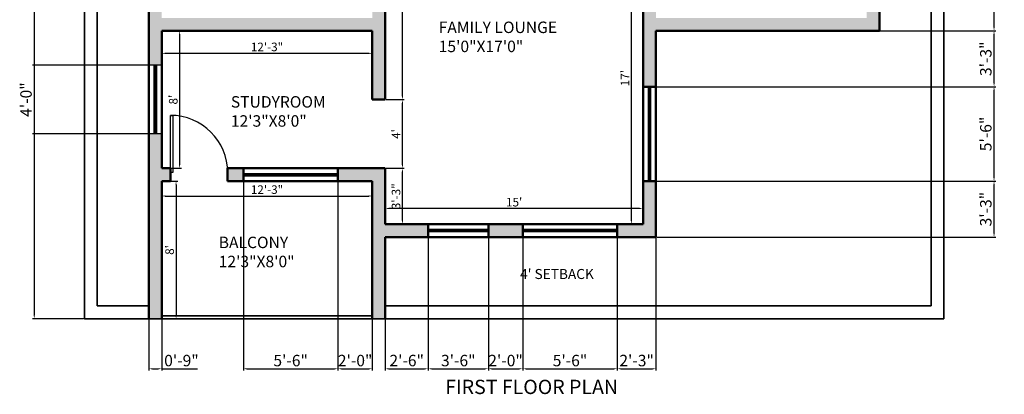
# Model space of a CAD drawing. Units: inches. Extents: x 2442 to 3851, y 589 to 2836.
# Tile 18 of 22: x 3164 to 3851, y 2138 to 2400. Entities that reach past the tile are written whole.
import ezdxf

# ---------------------------------------------------------------- set-up
doc = ezdxf.new("R2010")
doc.units = ezdxf.units.IN
for name, color, linetype, lineweight in [('A-ANNO-DIMS', 2, 'Continuous', 18), ('A-ANNO-TEXT', 7, 'Continuous', 18), ('A-AREA-IDEN', 7, 'Continuous', 18), ('A-DOOR', 4, 'Continuous', 25), ('A-GLAZ', 1, 'Continuous', 25), ('A-WALL', 7, 'Continuous', 50), ('A-WALL-PATT', 8, 'Continuous', 13), ('C-PROP', 7, 'Continuous', 35)]:
    doc.layers.add(name, color=color, linetype=linetype, lineweight=lineweight)
doc.styles.get("Standard").update_dxf_attribs({"font": 'arial.ttf'})
doc.dimstyles.new('ISO-25', dxfattribs={"dimtxt": 8, "dimasz": 2.5, "dimexe": 1.25, "dimexo": 0.625, "dimtad": 1, "dimlunit": 3, "dimtxsty": 'Standard', "dimcen": 2.5, "dimadec": 0, "dimazin": 0, "dimtfac": 1, "dimtmove": 0, "dimatfit": 3, "dimfxl": 1, "dimarcsym": 0})

# ---------------------------------------------------------------- blocks, each defined once
blk = doc.blocks.new('*U22')
for p, q in [((0, 0), (0, -6)), ((40, 0), (40, -6))]:
    blk.add_line(p, q)
blk.add_lwpolyline([(0, 0), (0, 40), (1.75, 40), (1.75, 0)], close=True)
blk.add_arc((0, 0), 40, 0, 90)
blk = doc.blocks.new('*D93')
at = {"layer": 'A-ANNO-DIMS', "color": 0, "lineweight": -2, "transparency": 16777216}
for p, q in [((3263.65, 2287.21), (3274.25, 2287.21)), ((3273, 2284.71), (3273, 2193.71)), ((3263.65, 2191.21), (3274.25, 2191.21))]:
    blk.add_line(p, q, dxfattribs=at)
at = {"layer": 'A-ANNO-DIMS', "color": 0, "transparency": 16777216}
for points in [[(3272.58, 2284.71), (3273.42, 2284.71), (3273, 2287.21)], [(3272.58, 2193.71), (3273.42, 2193.71), (3273, 2191.21)]]:
    blk.add_solid(points, dxfattribs=at)
at = {"layer": 'Defpoints', "color": 0, "transparency": 16777216}
for p in [(3263.02, 2287.21), (3263.02, 2191.21), (3273, 2191.21)]:
    blk.add_point(p, dxfattribs=at)
at = {"layer": 'A-ANNO-DIMS', "color": 0, "transparency": 16777216, "insert": (3269.31, 2239.21), "char_height": 6, "attachment_point": 5, "rotation": 90}
blk.add_mtext("8'", dxfattribs=at)
blk = doc.blocks.new('*D94')
at = {"layer": 'A-ANNO-DIMS', "color": 0, "lineweight": -2, "transparency": 16777216}
for p, q in [((3263.02, 2286.58), (3263.02, 2275.62)), ((3410.02, 2286.58), (3410.02, 2275.62)), ((3265.52, 2276.87), (3407.52, 2276.87))]:
    blk.add_line(p, q, dxfattribs=at)
at = {"layer": 'A-ANNO-DIMS', "color": 0, "transparency": 16777216}
for points in [[(3265.52, 2277.29), (3265.52, 2276.45), (3263.02, 2276.87)], [(3407.52, 2277.29), (3407.52, 2276.45), (3410.02, 2276.87)]]:
    blk.add_solid(points, dxfattribs=at)
at = {"layer": 'Defpoints', "color": 0, "transparency": 16777216}
for p in [(3263.02, 2287.21), (3410.02, 2287.21), (3410.02, 2276.87)]:
    blk.add_point(p, dxfattribs=at)
at = {"layer": 'A-ANNO-DIMS', "color": 0, "transparency": 16777216, "insert": (3336.52, 2280.56), "char_height": 6, "attachment_point": 5}
blk.add_mtext('12\'-3"', dxfattribs=at)
blk = doc.blocks.new('*D95')
at = {"layer": 'A-ANNO-DIMS', "color": 0, "lineweight": -2, "transparency": 16777216}
for p, q in [((3419.65, 2296.21), (3432.29, 2296.21)), ((3431.04, 2259.71), (3431.04, 2293.71)), ((3419.65, 2257.21), (3432.29, 2257.21))]:
    blk.add_line(p, q, dxfattribs=at)
at = {"layer": 'A-ANNO-DIMS', "color": 0, "transparency": 16777216}
for points in [[(3430.63, 2293.71), (3431.46, 2293.71), (3431.04, 2296.21)], [(3430.63, 2259.71), (3431.46, 2259.71), (3431.04, 2257.21)]]:
    blk.add_solid(points, dxfattribs=at)
at = {"layer": 'Defpoints', "color": 0, "transparency": 16777216}
for p in [(3419.02, 2296.21), (3431.04, 2296.21), (3419.02, 2257.21)]:
    blk.add_point(p, dxfattribs=at)
at = {"layer": 'A-ANNO-DIMS', "color": 0, "transparency": 16777216, "insert": (3427.35, 2276.71), "char_height": 6, "attachment_point": 5, "rotation": 90}
blk.add_mtext('3\'-3"', dxfattribs=at)
blk = doc.blocks.new('*D96')
at = {"layer": 'A-ANNO-DIMS', "color": 0, "lineweight": -2, "transparency": 16777216}
for p, q in [((3419.65, 2344.21), (3432.29, 2344.21)), ((3431.04, 2298.71), (3431.04, 2341.71)), ((3419.65, 2296.21), (3432.29, 2296.21))]:
    blk.add_line(p, q, dxfattribs=at)
at = {"layer": 'A-ANNO-DIMS', "color": 0, "transparency": 16777216}
for points in [[(3430.63, 2341.71), (3431.46, 2341.71), (3431.04, 2344.21)], [(3430.63, 2298.71), (3431.46, 2298.71), (3431.04, 2296.21)]]:
    blk.add_solid(points, dxfattribs=at)
at = {"layer": 'Defpoints', "color": 0, "transparency": 16777216}
for p in [(3419.02, 2344.21), (3431.04, 2344.21), (3419.02, 2296.21)]:
    blk.add_point(p, dxfattribs=at)
at = {"layer": 'A-ANNO-DIMS', "color": 0, "transparency": 16777216, "insert": (3427.42, 2320.21), "char_height": 6, "attachment_point": 5, "rotation": 90}
blk.add_mtext("4'", dxfattribs=at)
blk = doc.blocks.new('*D97')
at = {"layer": 'A-ANNO-DIMS', "color": 0, "lineweight": -2, "transparency": 16777216}
for p, q in [((3419.65, 2506.21), (3432.29, 2506.21)), ((3431.04, 2346.71), (3431.04, 2503.71)), ((3419.65, 2344.21), (3432.29, 2344.21))]:
    blk.add_line(p, q, dxfattribs=at)
at = {"layer": 'A-ANNO-DIMS', "color": 0, "transparency": 16777216}
for points in [[(3430.63, 2503.71), (3431.46, 2503.71), (3431.04, 2506.21)], [(3430.63, 2346.71), (3431.46, 2346.71), (3431.04, 2344.21)]]:
    blk.add_solid(points, dxfattribs=at)
at = {"layer": 'Defpoints', "color": 0, "transparency": 16777216}
for p in [(3419.02, 2506.21), (3431.04, 2506.21), (3419.02, 2344.21)]:
    blk.add_point(p, dxfattribs=at)
at = {"layer": 'A-ANNO-DIMS', "color": 0, "transparency": 16777216, "insert": (3427.35, 2425.21), "char_height": 6, "attachment_point": 5, "rotation": 90}
blk.add_mtext('13\'-6"', dxfattribs=at)
blk = doc.blocks.new('*D130')
at = {"layer": 'A-ANNO-DIMS', "color": 0, "lineweight": -2, "transparency": 16777216}
for p, q in [((3263.02, 2391.58), (3263.02, 2375.27)), ((3410.02, 2391.58), (3410.02, 2375.27)), ((3265.52, 2376.52), (3407.52, 2376.52))]:
    blk.add_line(p, q, dxfattribs=at)
at = {"layer": 'A-ANNO-DIMS', "color": 0, "transparency": 16777216}
for points in [[(3265.52, 2376.94), (3265.52, 2376.11), (3263.02, 2376.52)], [(3407.52, 2376.94), (3407.52, 2376.11), (3410.02, 2376.52)]]:
    blk.add_solid(points, dxfattribs=at)
at = {"layer": 'Defpoints', "color": 0, "transparency": 16777216}
for p in [(3263.02, 2392.21), (3410.02, 2392.21), (3410.02, 2376.52)]:
    blk.add_point(p, dxfattribs=at)
at = {"layer": 'A-ANNO-DIMS', "color": 0, "transparency": 16777216, "insert": (3336.52, 2380.21), "char_height": 6, "attachment_point": 5}
blk.add_mtext('12\'-3"', dxfattribs=at)
blk = doc.blocks.new('*D131')
at = {"layer": 'A-ANNO-DIMS', "color": 0, "lineweight": -2, "transparency": 16777216}
for p, q in [((3263.65, 2392.21), (3276.76, 2392.21)), ((3275.51, 2389.71), (3275.51, 2298.71)), ((3263.65, 2296.21), (3276.76, 2296.21))]:
    blk.add_line(p, q, dxfattribs=at)
at = {"layer": 'A-ANNO-DIMS', "color": 0, "transparency": 16777216}
for points in [[(3275.1, 2389.71), (3275.93, 2389.71), (3275.51, 2392.21)], [(3275.1, 2298.71), (3275.93, 2298.71), (3275.51, 2296.21)]]:
    blk.add_solid(points, dxfattribs=at)
at = {"layer": 'Defpoints', "color": 0, "transparency": 16777216}
for p in [(3263.02, 2392.21), (3263.02, 2296.21), (3275.51, 2296.21)]:
    blk.add_point(p, dxfattribs=at)
at = {"layer": 'A-ANNO-DIMS', "color": 0, "transparency": 16777216, "insert": (3271.82, 2344.21), "char_height": 6, "attachment_point": 5, "rotation": 90}
blk.add_mtext("8'", dxfattribs=at)
blk = doc.blocks.new('*D132')
at = {"layer": 'A-ANNO-DIMS', "color": 0, "lineweight": -2, "transparency": 16777216}
for p, q in [((3419.02, 2257.83), (3419.02, 2269.37)), ((3599.02, 2257.83), (3599.02, 2269.37)), ((3596.52, 2268.12), (3421.52, 2268.12))]:
    blk.add_line(p, q, dxfattribs=at)
at = {"layer": 'A-ANNO-DIMS', "color": 0, "transparency": 16777216}
for points in [[(3421.52, 2268.54), (3421.52, 2267.7), (3419.02, 2268.12)], [(3596.52, 2268.54), (3596.52, 2267.7), (3599.02, 2268.12)]]:
    blk.add_solid(points, dxfattribs=at)
at = {"layer": 'Defpoints', "color": 0, "transparency": 16777216}
for p in [(3419.02, 2268.12), (3419.02, 2257.21), (3599.02, 2257.21)]:
    blk.add_point(p, dxfattribs=at)
at = {"layer": 'A-ANNO-DIMS', "color": 0, "transparency": 16777216, "insert": (3509.02, 2271.81), "char_height": 6, "attachment_point": 5}
blk.add_mtext("15'", dxfattribs=at)
blk = doc.blocks.new('*D133')
at = {"layer": 'A-ANNO-DIMS', "color": 0, "lineweight": -2, "transparency": 16777216}
for p, q in [((3598.4, 2461.21), (3589.59, 2461.21)), ((3590.84, 2259.71), (3590.84, 2458.71)), ((3598.4, 2257.21), (3589.59, 2257.21))]:
    blk.add_line(p, q, dxfattribs=at)
at = {"layer": 'A-ANNO-DIMS', "color": 0, "transparency": 16777216}
for points in [[(3590.43, 2458.71), (3591.26, 2458.71), (3590.84, 2461.21)], [(3590.43, 2259.71), (3591.26, 2259.71), (3590.84, 2257.21)]]:
    blk.add_solid(points, dxfattribs=at)
at = {"layer": 'Defpoints', "color": 0, "transparency": 16777216}
for p in [(3590.84, 2461.21), (3599.02, 2461.21), (3599.02, 2257.21)]:
    blk.add_point(p, dxfattribs=at)
at = {"layer": 'A-ANNO-DIMS', "color": 0, "transparency": 16777216, "insert": (3587.21, 2359.21), "char_height": 6, "attachment_point": 5, "rotation": 90}
blk.add_mtext("17'", dxfattribs=at)
blk = doc.blocks.new('*D219')
at = {"layer": 'A-ANNO-DIMS', "color": 0, "lineweight": -2, "transparency": 16777216}
for p, q in [((3208.4, 2791.21), (3172.77, 2791.21)), ((3174.02, 2788.71), (3174.02, 2193.71)), ((3208.4, 2191.21), (3172.77, 2191.21))]:
    blk.add_line(p, q, dxfattribs=at)
at = {"layer": 'A-ANNO-DIMS', "color": 0, "transparency": 16777216}
for points in [[(3173.61, 2788.71), (3174.44, 2788.71), (3174.02, 2791.21)], [(3173.61, 2193.71), (3174.44, 2193.71), (3174.02, 2191.21)]]:
    blk.add_solid(points, dxfattribs=at)
at = {"layer": 'Defpoints', "color": 0, "transparency": 16777216}
for p in [(3209.02, 2791.21), (3174.02, 2191.21), (3209.02, 2191.21)]:
    blk.add_point(p, dxfattribs=at)
at = {"layer": 'A-ANNO-DIMS', "color": 0, "transparency": 16777216, "insert": (3169.31, 2491.21), "char_height": 8, "attachment_point": 5, "rotation": 90}
blk.add_mtext('50\'-0"', dxfattribs=at)
blk = doc.blocks.new('*D229')
at = {"layer": 'A-ANNO-DIMS', "color": 0, "lineweight": -2, "transparency": 16777216}
for p, q in [((3844.02, 2426.71), (3844.02, 2476.72)), ((3764.65, 2426.71), (3845.27, 2426.71)), ((3844.02, 2394.71), (3844.02, 2424.21)), ((3764.65, 2392.21), (3845.27, 2392.21))]:
    blk.add_line(p, q, dxfattribs=at)
at = {"layer": 'A-ANNO-DIMS', "color": 0, "transparency": 16777216}
for points in [[(3843.61, 2424.21), (3844.44, 2424.21), (3844.02, 2426.71)], [(3843.61, 2394.71), (3844.44, 2394.71), (3844.02, 2392.21)]]:
    blk.add_solid(points, dxfattribs=at)
at = {"layer": 'Defpoints', "color": 0, "transparency": 16777216}
for p in [(3764.02, 2426.71), (3844.02, 2426.71), (3764.02, 2392.21)]:
    blk.add_point(p, dxfattribs=at)
at = {"layer": 'A-ANNO-DIMS', "color": 0, "transparency": 16777216, "insert": (3839.26, 2452.96), "char_height": 8, "attachment_point": 5, "rotation": 90}
blk.add_mtext('2\'-10 1/2"', dxfattribs=at)
blk = doc.blocks.new('*D240')
at = {"layer": 'A-ANNO-DIMS', "color": 0, "lineweight": -2, "transparency": 16777216}
for p, q in [((3253.4, 2473.21), (3172.77, 2473.21)), ((3174.02, 2470.71), (3174.02, 2370.71)), ((3253.4, 2368.21), (3172.77, 2368.21))]:
    blk.add_line(p, q, dxfattribs=at)
at = {"layer": 'A-ANNO-DIMS', "color": 0, "transparency": 16777216}
for points in [[(3173.61, 2470.71), (3174.44, 2470.71), (3174.02, 2473.21)], [(3173.61, 2370.71), (3174.44, 2370.71), (3174.02, 2368.21)]]:
    blk.add_solid(points, dxfattribs=at)
at = {"layer": 'Defpoints', "color": 0, "transparency": 16777216}
for p in [(3254.02, 2473.21), (3174.02, 2368.21), (3254.02, 2368.21)]:
    blk.add_point(p, dxfattribs=at)
at = {"layer": 'A-ANNO-DIMS', "color": 0, "transparency": 16777216, "insert": (3169.31, 2420.71), "char_height": 8, "attachment_point": 5, "rotation": 90}
blk.add_mtext('8\'-9"', dxfattribs=at)
blk = doc.blocks.new('*D241')
at = {"layer": 'A-ANNO-DIMS', "color": 0, "lineweight": -2, "transparency": 16777216}
for p, q in [((3253.4, 2368.21), (3172.77, 2368.21)), ((3174.02, 2365.71), (3174.02, 2322.71)), ((3253.4, 2320.21), (3172.77, 2320.21))]:
    blk.add_line(p, q, dxfattribs=at)
at = {"layer": 'A-ANNO-DIMS', "color": 0, "transparency": 16777216}
for points in [[(3173.61, 2365.71), (3174.44, 2365.71), (3174.02, 2368.21)], [(3173.61, 2322.71), (3174.44, 2322.71), (3174.02, 2320.21)]]:
    blk.add_solid(points, dxfattribs=at)
at = {"layer": 'Defpoints', "color": 0, "transparency": 16777216}
for p in [(3254.02, 2368.21), (3174.02, 2320.21), (3254.02, 2320.21)]:
    blk.add_point(p, dxfattribs=at)
at = {"layer": 'A-ANNO-DIMS', "color": 0, "transparency": 16777216, "insert": (3169.31, 2344.21), "char_height": 8, "attachment_point": 5, "rotation": 90}
blk.add_mtext('4\'-0"', dxfattribs=at)
blk = doc.blocks.new('*D242')
at = {"layer": 'A-ANNO-DIMS', "color": 0, "lineweight": -2, "transparency": 16777216}
for p, q in [((3320.02, 2286.58), (3320.02, 2154.96)), ((3386.02, 2286.58), (3386.02, 2154.96)), ((3322.52, 2156.21), (3383.52, 2156.21))]:
    blk.add_line(p, q, dxfattribs=at)
at = {"layer": 'A-ANNO-DIMS', "color": 0, "transparency": 16777216}
for points in [[(3322.52, 2156.62), (3322.52, 2155.79), (3320.02, 2156.21)], [(3383.52, 2156.62), (3383.52, 2155.79), (3386.02, 2156.21)]]:
    blk.add_solid(points, dxfattribs=at)
at = {"layer": 'Defpoints', "color": 0, "transparency": 16777216}
for p in [(3320.02, 2287.21), (3386.02, 2287.21), (3386.02, 2156.21)]:
    blk.add_point(p, dxfattribs=at)
at = {"layer": 'A-ANNO-DIMS', "color": 0, "transparency": 16777216, "insert": (3353.02, 2160.92), "char_height": 8, "attachment_point": 5}
blk.add_mtext('5\'-6"', dxfattribs=at)
blk = doc.blocks.new('*D243')
at = {"layer": 'A-ANNO-DIMS', "color": 0, "lineweight": -2, "transparency": 16777216}
for p, q in [((3386.02, 2286.58), (3386.02, 2154.96)), ((3410.02, 2286.58), (3410.02, 2154.96)), ((3388.52, 2156.21), (3407.52, 2156.21))]:
    blk.add_line(p, q, dxfattribs=at)
at = {"layer": 'A-ANNO-DIMS', "color": 0, "transparency": 16777216}
for points in [[(3388.52, 2156.62), (3388.52, 2155.79), (3386.02, 2156.21)], [(3407.52, 2156.62), (3407.52, 2155.79), (3410.02, 2156.21)]]:
    blk.add_solid(points, dxfattribs=at)
at = {"layer": 'Defpoints', "color": 0, "transparency": 16777216}
for p in [(3386.02, 2287.21), (3410.02, 2287.21), (3410.02, 2156.21)]:
    blk.add_point(p, dxfattribs=at)
at = {"layer": 'A-ANNO-DIMS', "color": 0, "transparency": 16777216, "insert": (3398.02, 2160.92), "char_height": 8, "attachment_point": 5}
blk.add_mtext('2\'-0"', dxfattribs=at)
blk = doc.blocks.new('*D244')
at = {"layer": 'A-ANNO-DIMS', "color": 0, "lineweight": -2, "transparency": 16777216}
for p, q in [((3419.02, 2247.58), (3419.02, 2154.96)), ((3449.02, 2247.58), (3449.02, 2154.96)), ((3421.52, 2156.21), (3446.52, 2156.21))]:
    blk.add_line(p, q, dxfattribs=at)
at = {"layer": 'A-ANNO-DIMS', "color": 0, "transparency": 16777216}
for points in [[(3421.52, 2156.62), (3421.52, 2155.79), (3419.02, 2156.21)], [(3446.52, 2156.62), (3446.52, 2155.79), (3449.02, 2156.21)]]:
    blk.add_solid(points, dxfattribs=at)
at = {"layer": 'Defpoints', "color": 0, "transparency": 16777216}
for p in [(3419.02, 2248.21), (3449.02, 2248.21), (3449.02, 2156.21)]:
    blk.add_point(p, dxfattribs=at)
at = {"layer": 'A-ANNO-DIMS', "color": 0, "transparency": 16777216, "insert": (3434.02, 2160.92), "char_height": 8, "attachment_point": 5}
blk.add_mtext('2\'-6"', dxfattribs=at)
blk = doc.blocks.new('*D245')
at = {"layer": 'A-ANNO-DIMS', "color": 0, "lineweight": -2, "transparency": 16777216}
for p, q in [((3449.02, 2247.58), (3449.02, 2154.96)), ((3491.02, 2247.58), (3491.02, 2154.96)), ((3451.52, 2156.21), (3488.52, 2156.21))]:
    blk.add_line(p, q, dxfattribs=at)
at = {"layer": 'A-ANNO-DIMS', "color": 0, "transparency": 16777216}
for points in [[(3451.52, 2156.62), (3451.52, 2155.79), (3449.02, 2156.21)], [(3488.52, 2156.62), (3488.52, 2155.79), (3491.02, 2156.21)]]:
    blk.add_solid(points, dxfattribs=at)
at = {"layer": 'Defpoints', "color": 0, "transparency": 16777216}
for p in [(3449.02, 2248.21), (3491.02, 2248.21), (3491.02, 2156.21)]:
    blk.add_point(p, dxfattribs=at)
at = {"layer": 'A-ANNO-DIMS', "color": 0, "transparency": 16777216, "insert": (3470.02, 2160.92), "char_height": 8, "attachment_point": 5}
blk.add_mtext('3\'-6"', dxfattribs=at)
blk = doc.blocks.new('*D246')
at = {"layer": 'A-ANNO-DIMS', "color": 0, "lineweight": -2, "transparency": 16777216}
for p, q in [((3491.02, 2247.58), (3491.02, 2154.96)), ((3515.02, 2247.58), (3515.02, 2154.96)), ((3493.52, 2156.21), (3512.52, 2156.21))]:
    blk.add_line(p, q, dxfattribs=at)
at = {"layer": 'A-ANNO-DIMS', "color": 0, "transparency": 16777216}
for points in [[(3493.52, 2156.62), (3493.52, 2155.79), (3491.02, 2156.21)], [(3512.52, 2156.62), (3512.52, 2155.79), (3515.02, 2156.21)]]:
    blk.add_solid(points, dxfattribs=at)
at = {"layer": 'Defpoints', "color": 0, "transparency": 16777216}
for p in [(3491.02, 2248.21), (3515.02, 2248.21), (3515.02, 2156.21)]:
    blk.add_point(p, dxfattribs=at)
at = {"layer": 'A-ANNO-DIMS', "color": 0, "transparency": 16777216, "insert": (3503.02, 2160.92), "char_height": 8, "attachment_point": 5}
blk.add_mtext('2\'-0"', dxfattribs=at)
blk = doc.blocks.new('*D247')
at = {"layer": 'A-ANNO-DIMS', "color": 0, "lineweight": -2, "transparency": 16777216}
for p, q in [((3515.02, 2247.58), (3515.02, 2154.96)), ((3581.02, 2247.58), (3581.02, 2154.96)), ((3517.52, 2156.21), (3578.52, 2156.21))]:
    blk.add_line(p, q, dxfattribs=at)
at = {"layer": 'A-ANNO-DIMS', "color": 0, "transparency": 16777216}
for points in [[(3517.52, 2156.62), (3517.52, 2155.79), (3515.02, 2156.21)], [(3578.52, 2156.62), (3578.52, 2155.79), (3581.02, 2156.21)]]:
    blk.add_solid(points, dxfattribs=at)
at = {"layer": 'Defpoints', "color": 0, "transparency": 16777216}
for p in [(3515.02, 2248.21), (3581.02, 2248.21), (3581.02, 2156.21)]:
    blk.add_point(p, dxfattribs=at)
at = {"layer": 'A-ANNO-DIMS', "color": 0, "transparency": 16777216, "insert": (3548.02, 2160.92), "char_height": 8, "attachment_point": 5}
blk.add_mtext('5\'-6"', dxfattribs=at)
blk = doc.blocks.new('*D248')
at = {"layer": 'A-ANNO-DIMS', "color": 0, "lineweight": -2, "transparency": 16777216}
for p, q in [((3581.02, 2247.58), (3581.02, 2154.96)), ((3608.02, 2247.58), (3608.02, 2154.96)), ((3583.52, 2156.21), (3605.52, 2156.21))]:
    blk.add_line(p, q, dxfattribs=at)
at = {"layer": 'A-ANNO-DIMS', "color": 0, "transparency": 16777216}
for points in [[(3583.52, 2156.62), (3583.52, 2155.79), (3581.02, 2156.21)], [(3605.52, 2156.62), (3605.52, 2155.79), (3608.02, 2156.21)]]:
    blk.add_solid(points, dxfattribs=at)
at = {"layer": 'Defpoints', "color": 0, "transparency": 16777216}
for p in [(3581.02, 2248.21), (3608.02, 2248.21), (3608.02, 2156.21)]:
    blk.add_point(p, dxfattribs=at)
at = {"layer": 'A-ANNO-DIMS', "color": 0, "transparency": 16777216, "insert": (3594.52, 2160.92), "char_height": 8, "attachment_point": 5}
blk.add_mtext('2\'-3"', dxfattribs=at)
blk = doc.blocks.new('*D249')
at = {"layer": 'A-ANNO-DIMS', "color": 0, "lineweight": -2, "transparency": 16777216}
for p, q in [((3608.65, 2287.21), (3845.27, 2287.21)), ((3844.02, 2250.71), (3844.02, 2284.71)), ((3608.65, 2248.21), (3845.27, 2248.21))]:
    blk.add_line(p, q, dxfattribs=at)
at = {"layer": 'A-ANNO-DIMS', "color": 0, "transparency": 16777216}
for points in [[(3843.61, 2284.71), (3844.44, 2284.71), (3844.02, 2287.21)], [(3843.61, 2250.71), (3844.44, 2250.71), (3844.02, 2248.21)]]:
    blk.add_solid(points, dxfattribs=at)
at = {"layer": 'Defpoints', "color": 0, "transparency": 16777216}
for p in [(3608.02, 2287.21), (3844.02, 2287.21), (3608.02, 2248.21)]:
    blk.add_point(p, dxfattribs=at)
at = {"layer": 'A-ANNO-DIMS', "color": 0, "transparency": 16777216, "insert": (3839.31, 2267.71), "char_height": 8, "attachment_point": 5, "rotation": 90}
blk.add_mtext('3\'-3"', dxfattribs=at)
blk = doc.blocks.new('*D250')
at = {"layer": 'A-ANNO-DIMS', "color": 0, "lineweight": -2, "transparency": 16777216}
for p, q in [((3608.65, 2353.21), (3845.27, 2353.21)), ((3844.02, 2289.71), (3844.02, 2350.71)), ((3608.65, 2287.21), (3845.27, 2287.21))]:
    blk.add_line(p, q, dxfattribs=at)
at = {"layer": 'A-ANNO-DIMS', "color": 0, "transparency": 16777216}
for points in [[(3843.61, 2350.71), (3844.44, 2350.71), (3844.02, 2353.21)], [(3843.61, 2289.71), (3844.44, 2289.71), (3844.02, 2287.21)]]:
    blk.add_solid(points, dxfattribs=at)
at = {"layer": 'Defpoints', "color": 0, "transparency": 16777216}
for p in [(3608.02, 2353.21), (3844.02, 2353.21), (3608.02, 2287.21)]:
    blk.add_point(p, dxfattribs=at)
at = {"layer": 'A-ANNO-DIMS', "color": 0, "transparency": 16777216, "insert": (3839.31, 2320.21), "char_height": 8, "attachment_point": 5, "rotation": 90}
blk.add_mtext('5\'-6"', dxfattribs=at)
blk = doc.blocks.new('*D251')
at = {"layer": 'A-ANNO-DIMS', "color": 0, "lineweight": -2, "transparency": 16777216}
for p, q in [((3608.65, 2392.21), (3845.27, 2392.21)), ((3844.02, 2355.71), (3844.02, 2389.71)), ((3608.65, 2353.21), (3845.27, 2353.21))]:
    blk.add_line(p, q, dxfattribs=at)
at = {"layer": 'A-ANNO-DIMS', "color": 0, "transparency": 16777216}
for points in [[(3843.61, 2389.71), (3844.44, 2389.71), (3844.02, 2392.21)], [(3843.61, 2355.71), (3844.44, 2355.71), (3844.02, 2353.21)]]:
    blk.add_solid(points, dxfattribs=at)
at = {"layer": 'Defpoints', "color": 0, "transparency": 16777216}
for p in [(3608.02, 2392.21), (3844.02, 2392.21), (3608.02, 2353.21)]:
    blk.add_point(p, dxfattribs=at)
at = {"layer": 'A-ANNO-DIMS', "color": 0, "transparency": 16777216, "insert": (3839.31, 2372.71), "char_height": 8, "attachment_point": 5, "rotation": 90}
blk.add_mtext('3\'-3"', dxfattribs=at)
blk = doc.blocks.new('*D252')
at = {"layer": 'A-ANNO-DIMS', "color": 0, "lineweight": -2, "transparency": 16777216}
for p, q in [((3254.02, 2190.58), (3254.02, 2154.96)), ((3263.02, 2190.58), (3263.02, 2154.96)), ((3256.52, 2156.21), (3260.52, 2156.21)), ((3263.02, 2156.21), (3288.04, 2156.21))]:
    blk.add_line(p, q, dxfattribs=at)
at = {"layer": 'A-ANNO-DIMS', "color": 0, "transparency": 16777216}
for points in [[(3256.52, 2156.62), (3256.52, 2155.79), (3254.02, 2156.21)], [(3260.52, 2156.62), (3260.52, 2155.79), (3263.02, 2156.21)]]:
    blk.add_solid(points, dxfattribs=at)
at = {"layer": 'Defpoints', "color": 0, "transparency": 16777216}
for p in [(3254.02, 2191.21), (3263.02, 2191.21), (3263.02, 2156.21)]:
    blk.add_point(p, dxfattribs=at)
at = {"layer": 'A-ANNO-DIMS', "color": 0, "transparency": 16777216, "insert": (3276.78, 2160.92), "char_height": 8, "attachment_point": 5}
blk.add_mtext('0\'-9"', dxfattribs=at)

msp = doc.modelspace()

# ---------------------------------------------------------------- hatches: boundary and pattern name
at = {"layer": 'A-WALL-PATT'}
h = msp.add_hatch(color=256, dxfattribs=at)
h.dxf.hatch_style = 1
h.paths.add_polyline_path([(3356.024, 2713.208), (3356.024, 2719.208), (3356.024, 2722.208), (3254.024, 2722.208), (3254.024, 2657.708), (3263.024, 2657.708), (3263.024, 2713.208)])
h.paths.add_polyline_path([(3416.024, 2737.208), (3446.024, 2737.208), (3446.024, 2746.208), (3416.024, 2746.208), (3416.024, 2782.208), (3407.024, 2782.208), (3407.024, 2722.208), (3386.024, 2722.208), (3386.024, 2719.208), (3386.024, 2713.208), (3407.024, 2713.208), (3407.024, 2593.208), (3416.024, 2593.208), (3416.024, 2608.208), (3515.024, 2608.208), (3515.024, 2614.208), (3515.024, 2617.208), (3416.024, 2617.208)])
h.paths.add_polyline_path([(3563.024, 2737.208), (3566.024, 2737.208), (3566.024, 2746.208), (3512.024, 2746.208), (3512.024, 2737.208), (3554.024, 2737.208), (3554.024, 2617.208), (3551.024, 2617.208), (3551.024, 2614.208), (3551.024, 2608.208), (3554.024, 2608.208), (3554.024, 2554.208), (3566.024, 2554.208), (3566.024, 2560.208), (3566.024, 2563.208), (3563.024, 2563.208)])
h.paths.add_polyline_path([(3614.024, 2746.208), (3614.024, 2737.208), (3683.024, 2737.208), (3683.024, 2746.208)])
h.paths.add_polyline_path([(3755.024, 2737.208), (3755.024, 2665.208), (3764.024, 2665.208), (3764.024, 2746.208), (3731.024, 2746.208), (3731.024, 2737.208)])
h.paths.add_polyline_path([(3662.024, 2617.208), (3662.024, 2611.208), (3755.024, 2611.208), (3755.024, 2605.208), (3764.024, 2605.208), (3764.024, 2617.208)])
h.paths.add_polyline_path([(3755.024, 2554.208), (3755.024, 2548.208), (3764.024, 2548.208), (3764.024, 2569.208), (3755.024, 2569.208), (3755.024, 2563.208), (3677.024, 2563.208), (3677.024, 2581.208), (3671.024, 2581.208), (3671.024, 2563.208), (3611.024, 2563.208), (3611.024, 2611.208), (3632.024, 2611.208), (3632.024, 2617.208), (3605.024, 2617.208), (3605.024, 2563.208), (3602.024, 2563.208), (3602.024, 2554.208), (3653.024, 2554.208), (3653.024, 2536.208), (3659.024, 2536.208), (3659.024, 2554.208)])
h.paths.add_polyline_path([(3764.024, 2512.208), (3755.024, 2512.208), (3755.024, 2506.208), (3653.024, 2506.208), (3653.024, 2500.208), (3755.024, 2500.208), (3755.024, 2474.708), (3764.024, 2474.708)])
h.paths.add_polyline_path([(3608.024, 2392.208), (3764.024, 2392.208), (3764.024, 2426.708), (3755.024, 2426.708), (3755.024, 2401.208), (3608.024, 2401.208), (3608.024, 2461.208), (3599.024, 2461.208), (3599.024, 2353.208), (3608.024, 2353.208)])
h.paths.add_polyline_path([(3410.024, 2401.208), (3263.024, 2401.208), (3263.024, 2473.208), (3254.024, 2473.208), (3254.024, 2368.208), (3263.024, 2368.208), (3263.024, 2392.208), (3410.024, 2392.208), (3410.024, 2344.208), (3419.024, 2344.208), (3419.024, 2506.208), (3413.024, 2506.208), (3410.024, 2506.208)])
h.paths.add_polyline_path([(3263.024, 2609.708), (3254.024, 2609.708), (3254.024, 2521.208), (3263.024, 2521.208), (3263.024, 2545.208), (3410.024, 2545.208), (3410.024, 2542.208), (3413.024, 2542.208), (3419.024, 2542.208), (3419.024, 2557.208), (3407.024, 2557.208), (3407.024, 2554.208), (3263.024, 2554.208)])
h.paths.add_polyline_path([(3254.024, 2191.208), (3263.024, 2191.208), (3263.024, 2287.208), (3269.024, 2287.208), (3269.024, 2293.208), (3269.024, 2296.208), (3263.024, 2296.208), (3263.024, 2320.208), (3254.024, 2320.208)])
h.paths.add_polyline_path([(3419.024, 2296.208), (3386.024, 2296.208), (3386.024, 2287.208), (3410.024, 2287.208), (3410.024, 2191.208), (3419.024, 2191.208), (3419.024, 2248.208), (3449.024, 2248.208), (3449.024, 2257.208), (3419.024, 2257.208)])
h.paths.add_polyline_path([(3581.024, 2248.208), (3608.024, 2248.208), (3608.024, 2287.208), (3599.024, 2287.208), (3599.024, 2257.208), (3581.024, 2257.208)])
h.paths.add_polyline_path([(3491.024, 2248.208), (3515.024, 2248.208), (3515.024, 2257.208), (3491.024, 2257.208)])
h.paths.add_polyline_path([(3320.024, 2296.208), (3309.024, 2296.208), (3309.024, 2287.208), (3320.024, 2287.208)])
h.paths.add_polyline_path([(3282.007, 2631.263), (3387.059, 2631.263), (3387.059, 2661.678), (3282.007, 2661.678)], flags=9)
h.paths.add_polyline_path([(3511.253, 2214.916), (3571.545, 2214.916), (3571.545, 2229.862), (3511.253, 2229.862)], flags=9)
h.paths.add_polyline_path([(3777.335, 2589.915), (3777.335, 2529.623), (3792.281, 2529.623), (3792.281, 2589.915)], flags=9)
h.paths.add_polyline_path([(3558.97, 2754.629), (3619.262, 2754.629), (3619.262, 2769.575), (3558.97, 2769.575)], flags=9)
h.paths.add_polyline_path([(3314.979, 2749.318), (3377.263, 2749.318), (3377.263, 2779.733), (3314.979, 2779.733)], flags=9)
h.paths.add_polyline_path([(3624.453, 2577.252), (3671.045, 2577.252), (3671.045, 2600.063), (3624.453, 2600.063)], flags=25)
h.paths.add_polyline_path([(3701.15, 2577.252), (3744.07, 2577.252), (3744.07, 2600.063), (3701.15, 2600.063)], flags=25)
h.paths.add_polyline_path([(3689.533, 2518.545), (3731.868, 2518.545), (3731.868, 2541.356), (3689.533, 2541.356)], flags=9)
h.paths.add_polyline_path([(3629.196, 2666.979), (3693.452, 2666.979), (3693.452, 2697.394), (3629.196, 2697.394)], flags=9)
h.paths.add_polyline_path([(3441.284, 2669.891), (3505.54, 2669.891), (3505.54, 2700.306), (3441.284, 2700.306)], flags=25)
h.paths.add_polyline_path([(3306.565, 2459.233), (3370.821, 2459.233), (3370.821, 2489.648), (3306.565, 2489.648)], flags=25)
h.paths.add_polyline_path([(3307.889, 2320.733), (3387.355, 2320.733), (3387.355, 2351.148), (3307.889, 2351.148)], flags=9)
h.paths.add_polyline_path([(3452.987, 2372.794), (3554.971, 2372.794), (3554.971, 2403.208), (3452.987, 2403.208)], flags=9)

# ---------------------------------------------------------------- linework, layer by layer
at = {"layer": 'A-GLAZ'}
for p, q in [((3263.024, 2368.208), (3254.024, 2368.208)), ((3263.024, 2320.208), (3254.024, 2320.208))]:
    msp.add_line(p, q, dxfattribs=at)
at = {"layer": 'A-WALL'}
for p, q in [((3254.024, 2782.208), (3254.024, 2191.208)), ((3764.024, 2392.208), (3764.024, 2746.208)), ((3419.024, 2344.208), (3419.024, 2506.208)), ((3599.024, 2257.208), (3599.024, 2461.208)), ((3263.024, 2392.208), (3263.024, 2296.208)), ((3263.024, 2392.208), (3410.024, 2392.208)), ((3410.024, 2344.208), (3410.024, 2392.208)), ((3608.024, 2248.208), (3608.024, 2392.208)), ((3608.024, 2392.208), (3764.024, 2392.208)), ((3258.024, 2368.208), (3258.024, 2320.208)), ((3259.024, 2368.208), (3259.024, 2320.208)), ((3599.024, 2353.208), (3608.024, 2353.208)), ((3603.024, 2287.208), (3603.024, 2353.208)), ((3604.024, 2287.208), (3604.024, 2353.208)), ((3410.024, 2344.208), (3419.024, 2344.208)), ((3263.024, 2296.208), (3269.024, 2296.208)), ((3269.024, 2296.208), (3269.024, 2287.208)), ((3309.024, 2296.208), (3309.024, 2287.208)), ((3309.024, 2296.208), (3419.024, 2296.208)), ((3320.024, 2287.208), (3320.024, 2296.208)), ((3386.024, 2287.208), (3386.024, 2296.208)), ((3419.024, 2257.208), (3419.024, 2296.208)), ((3320.024, 2292.208), (3386.024, 2292.208)), ((3320.024, 2291.208), (3386.024, 2291.208)), ((3263.024, 2287.208), (3263.024, 2191.208)), ((3263.024, 2287.208), (3269.024, 2287.208)), ((3309.024, 2287.208), (3410.024, 2287.208)), ((3410.024, 2191.208), (3410.024, 2287.208)), ((3599.024, 2287.208), (3608.024, 2287.208)), ((3419.024, 2257.208), (3599.024, 2257.208)), ((3449.024, 2248.208), (3449.024, 2257.208)), ((3491.024, 2248.208), (3491.024, 2257.208)), ((3515.024, 2248.208), (3515.024, 2257.208)), ((3581.024, 2248.208), (3581.024, 2257.208)), ((3419.024, 2248.208), (3608.024, 2248.208)), ((3419.024, 2191.208), (3419.024, 2248.208)), ((3449.024, 2253.208), (3491.024, 2253.208)), ((3449.024, 2252.208), (3491.024, 2252.208)), ((3515.024, 2253.208), (3581.024, 2253.208)), ((3515.024, 2252.208), (3581.024, 2252.208))]:
    msp.add_line(p, q, dxfattribs=at)
at = {"layer": 'C-PROP'}
for points in [[(3809.024, 2191.208), (3809.024, 2791.208), (3209.024, 2791.208), (3209.024, 2191.208), (3809.024, 2191.208)], [(3800.024, 2200.208), (3800.024, 2782.208), (3218.024, 2782.208), (3218.024, 2200.208), (3254.024, 2200.208)], [(3419.024, 2200.208), (3800.024, 2200.208)], [(3263.024, 2193.208), (3410.024, 2193.208)]]:
    msp.add_lwpolyline(points, dxfattribs=at)

# ---------------------------------------------------------------- block references
at = {"layer": 'A-DOOR'}
msp.add_blockref('*U22', (3269.024, 2293.208), dxfattribs=at)

# ---------------------------------------------------------------- texts
at = {"layer": 'A-ANNO-TEXT', "attachment_point": 1}
for s, width, insert, char_height in [("{\\fTimes New Roman|b0|i0|c0|p18;4' SETBACK}", 79.56037, (3513.164, 2225.902), 7), ('{\\fTimes New Roman|b0|i0|c0|p18;FIRST FLOOR PLAN}', 196.26071, (3460.903, 2148.561), 10)]:
    msp.add_mtext_dynamic_manual_height_columns(s, width=width, gutter_width=12.5, heights=[0], dxfattribs=dict(at, insert=insert, char_height=char_height))
at = {"layer": 'A-AREA-IDEN', "char_height": 8, "attachment_point": 1}
for s, insert in [('{\\fTimes New Roman|b0|i0|c0|p18;FAMILY LOUNGE\\P15\'0"X17\'0"}', (3456.372, 2398.682)), ('{\\fTimes New Roman|b0|i0|c0|p18;STUDYROOM\\P12\'3"X8\'0"}', (3311.273, 2346.621)), ('{\\fTimes New Roman|b0|i0|c0|p18;BALCONY\\P12\'3"X8\'0"}', (3302.804, 2248.465))]:
    msp.add_mtext_dynamic_manual_height_columns(s, width=110.76054, gutter_width=12.5, heights=[0], dxfattribs=dict(at, insert=insert))

# ---------------------------------------------------------------- dimensions: what is measured, and where the dimension line sits
at = {"layer": 'A-ANNO-DIMS'}
for base, p1, p2, override, picture, middle in [((3174.024, 2191.208), (3209.024, 2791.208), (3209.024, 2191.208), {"dimdec": 1, "dimlfac": 1, "dimrnd": 0, "dimzin": 1, "dimdsep": 46, "dimlunit": 4, "dimfrac": 2}, '*D219', (3169.315, 2491.208)), ((3431.044, 2506.208), (3419.024, 2344.208), (3419.024, 2506.208), {"dimtxt": 6, "dimclrd": 0, "dimclre": 0, "dimclrt": 0, "dimtmove": 1}, '*D97', (3427.353, 2425.208)), ((3844.024, 2426.708), (3764.024, 2392.208), (3764.024, 2426.708), {"dimdec": 1, "dimlfac": 1, "dimrnd": 0, "dimzin": 1, "dimdsep": 46, "dimlunit": 4, "dimfrac": 2}, '*D229', (3839.263, 2452.962)), ((3174.024, 2368.208), (3254.024, 2473.208), (3254.024, 2368.208), {"dimdec": 1, "dimlfac": 1, "dimrnd": 0, "dimzin": 1, "dimdsep": 46, "dimlunit": 4, "dimfrac": 2}, '*D240', (3169.315, 2420.708)), ((3590.844, 2461.208), (3599.024, 2257.208), (3599.024, 2461.208), {"dimtxt": 6, "dimclrd": 0, "dimclre": 0, "dimclrt": 0}, '*D133', (3587.207, 2359.208)), ((3275.512, 2296.208), (3263.024, 2392.208), (3263.024, 2296.208), {"dimtxt": 6, "dimclrd": 0, "dimclre": 0, "dimclrt": 0}, '*D131', (3271.824, 2344.208)), ((3844.024, 2392.208), (3608.024, 2353.208), (3608.024, 2392.208), {"dimdec": 1, "dimlfac": 1, "dimrnd": 0, "dimzin": 1, "dimdsep": 46, "dimlunit": 4, "dimfrac": 2}, '*D251', (3839.312, 2372.708)), ((3174.024, 2320.208), (3254.024, 2368.208), (3254.024, 2320.208), {"dimdec": 1, "dimlfac": 1, "dimrnd": 0, "dimzin": 1, "dimdsep": 46, "dimlunit": 4, "dimfrac": 2}, '*D241', (3169.315, 2344.208)), ((3844.024, 2353.208), (3608.024, 2287.208), (3608.024, 2353.208), {"dimdec": 1, "dimlfac": 1, "dimrnd": 0, "dimzin": 1, "dimdsep": 46, "dimlunit": 4, "dimfrac": 2}, '*D250', (3839.315, 2320.208)), ((3431.044, 2344.208), (3419.024, 2296.208), (3419.024, 2344.208), {"dimtxt": 6, "dimclrd": 0, "dimclre": 0, "dimclrt": 0, "dimtmove": 1}, '*D96', (3427.419, 2320.208)), ((3431.044, 2296.208), (3419.024, 2257.208), (3419.024, 2296.208), {"dimtxt": 6, "dimclrd": 0, "dimclre": 0, "dimclrt": 0}, '*D95', (3427.353, 2276.708)), ((3273.002, 2191.208), (3263.024, 2287.208), (3263.024, 2191.208), {"dimtxt": 6, "dimclrd": 0, "dimclre": 0, "dimclrt": 0}, '*D93', (3269.313, 2239.208)), ((3844.024, 2287.208), (3608.024, 2248.208), (3608.024, 2287.208), {"dimdec": 1, "dimlfac": 1, "dimrnd": 0, "dimzin": 1, "dimdsep": 46, "dimlunit": 4, "dimfrac": 2}, '*D249', (3839.312, 2267.708))]:
    dim = msp.add_linear_dim(base=base, p1=p1, p2=p2, angle=90, dimstyle='ISO-25', override=override, dxfattribs=at)
    dim.commit()
    dim.dimension.update_dxf_attribs({"geometry": picture, "text_midpoint": middle})
for base, p1, p2, override, picture, middle in [((3410.024, 2376.524), (3263.024, 2392.208), (3410.024, 2392.208), {"dimtxt": 6, "dimclrd": 0, "dimclre": 0, "dimclrt": 0}, '*D130', (3336.524, 2380.214)), ((3410.024, 2276.871), (3263.024, 2287.208), (3410.024, 2287.208), {"dimtxt": 6, "dimclrd": 0, "dimclre": 0, "dimclrt": 0}, '*D94', (3336.524, 2280.561)), ((3386.024, 2156.208), (3320.024, 2287.208), (3386.024, 2287.208), {"dimdec": 1, "dimlfac": 1, "dimrnd": 0, "dimzin": 1, "dimdsep": 46, "dimlunit": 4, "dimfrac": 2}, '*D242', (3353.024, 2160.917)), ((3410.024, 2156.208), (3386.024, 2287.208), (3410.024, 2287.208), {"dimdec": 1, "dimlfac": 1, "dimrnd": 0, "dimzin": 1, "dimdsep": 46, "dimlunit": 4, "dimfrac": 2}, '*D243', (3398.024, 2160.917)), ((3419.024, 2268.121), (3599.024, 2257.208), (3419.024, 2257.208), {"dimtxt": 6, "dimclrd": 0, "dimclre": 0, "dimclrt": 0}, '*D132', (3509.024, 2271.809)), ((3449.024, 2156.208), (3419.024, 2248.208), (3449.024, 2248.208), {"dimdec": 1, "dimlfac": 1, "dimrnd": 0, "dimzin": 1, "dimdsep": 46, "dimlunit": 4, "dimfrac": 2}, '*D244', (3434.024, 2160.917)), ((3491.024, 2156.208), (3449.024, 2248.208), (3491.024, 2248.208), {"dimdec": 1, "dimlfac": 1, "dimrnd": 0, "dimzin": 1, "dimdsep": 46, "dimlunit": 4, "dimfrac": 2}, '*D245', (3470.024, 2160.92)), ((3515.024, 2156.208), (3491.024, 2248.208), (3515.024, 2248.208), {"dimdec": 1, "dimlfac": 1, "dimrnd": 0, "dimzin": 1, "dimdsep": 46, "dimlunit": 4, "dimfrac": 2}, '*D246', (3503.024, 2160.917)), ((3581.024, 2156.208), (3515.024, 2248.208), (3581.024, 2248.208), {"dimdec": 1, "dimlfac": 1, "dimrnd": 0, "dimzin": 1, "dimdsep": 46, "dimlunit": 4, "dimfrac": 2}, '*D247', (3548.024, 2160.917)), ((3608.024, 2156.208), (3581.024, 2248.208), (3608.024, 2248.208), {"dimdec": 1, "dimlfac": 1, "dimrnd": 0, "dimzin": 1, "dimdsep": 46, "dimlunit": 4, "dimfrac": 2}, '*D248', (3594.524, 2160.92)), ((3263.024, 2156.208), (3254.024, 2191.208), (3263.024, 2191.208), {"dimdec": 1, "dimlfac": 1, "dimrnd": 0, "dimzin": 1, "dimdsep": 46, "dimlunit": 4, "dimfrac": 2}, '*D252', (3276.783, 2160.917))]:
    dim = msp.add_linear_dim(base=base, p1=p1, p2=p2, dimstyle='ISO-25', override=override, dxfattribs=at)
    dim.commit()
    dim.dimension.update_dxf_attribs({"geometry": picture, "text_midpoint": middle})

doc.saveas('drawing.dxf')
